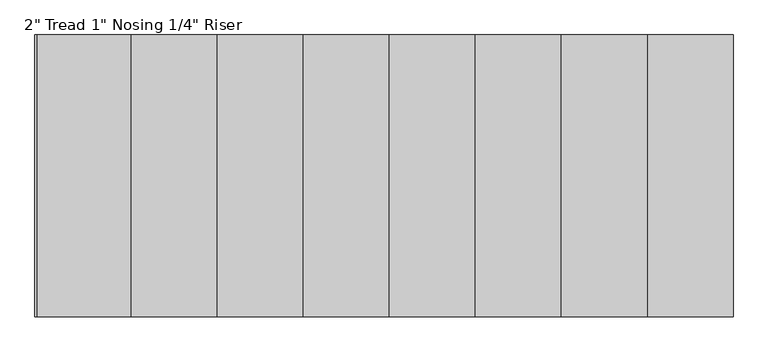
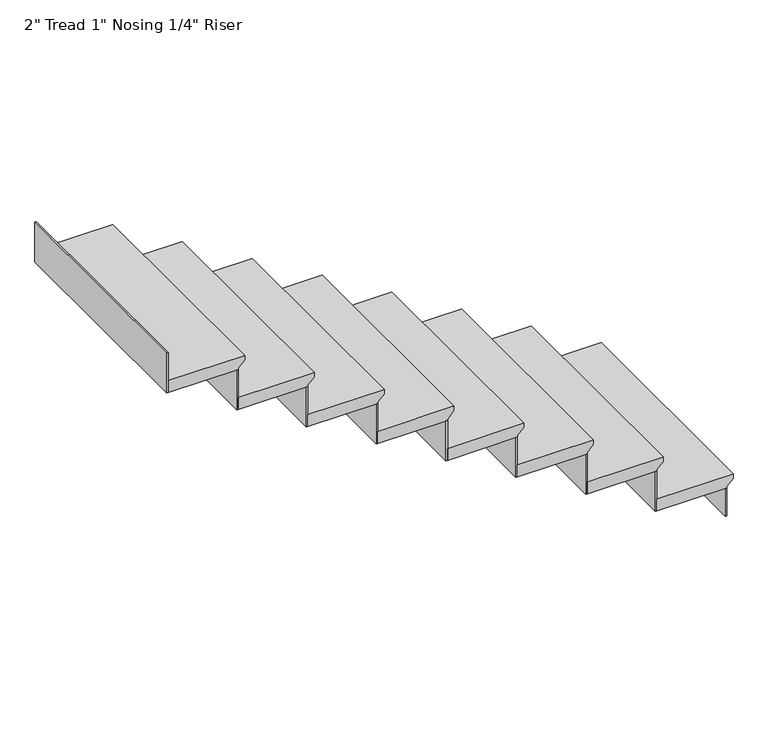
"""IFC4 building model written with IfcOpenShell, lengths in millimetres: stair flight geometry."""

from ifc_helpers import new_model, si_unit, origin, place, context, project, spatial, faceted_brep, source, transform, mapped, element, save


def stair_flight_6609341a(model_context):
    return source(origin(), model_context, "Body", "Brep", [
        faceted_brep([(-7578.3920073, 4811.1398463, 150.2833333), (-7578.3920073, 4811.1398463, 169.3333333), (-7578.3920073, 3896.7398463, 169.3333333), (-7578.3920073, 3896.7398463, 150.2833333), (-7603.7920073, 4811.1398463, 124.8833333), (-7603.7920073, 3896.7398463, 124.8833333), (-7883.1920073, 4811.1398463, 169.3333333), (-7883.1920073, 3896.7398463, 169.3333333), (-7603.7920073, 3896.7398463, 118.5333333), (-7883.1920073, 3896.7398463, 118.5333333), (-7883.1920073, 4811.1398463, 118.5333333), (-7603.7920073, 4811.1398463, 118.5333333)], [[[0, 1, 2, 3]], [[4, 0, 3, 5]], [[2, 1, 6, 7]], [[8, 9, 10, 11]], [[2, 7, 9, 8, 5, 3]], [[8, 11, 4, 5]], [[6, 1, 0, 4, 11, 10]], [[7, 6, 10, 9]]]),
        faceted_brep([(-7603.7920073, 4811.1398463, 118.5333333), (-7603.7920073, 4811.1398463, 0.0), (-7610.1420073, 4811.1398463, 0.0), (-7610.1420073, 4811.1398463, 118.5333333), (-7603.7920073, 3896.7398463, 118.5333333), (-7610.1420073, 3896.7398463, 118.5333333), (-7610.1420073, 3896.7398463, 0.0), (-7603.7920073, 3896.7398463, 0.0)], [[[0, 1, 2, 3]], [[4, 5, 6, 7]], [[1, 0, 4, 7]], [[2, 1, 7, 6]], [[3, 2, 6, 5]], [[0, 3, 5, 4]]]),
        faceted_brep([(-7883.1920073, 4811.1398463, 287.8666667), (-7883.1920073, 4811.1398463, 118.5333333), (-7889.5420073, 4811.1398463, 118.5333333), (-7889.5420073, 4811.1398463, 287.8666667), (-7883.1920073, 3896.7398463, 287.8666667), (-7889.5420073, 3896.7398463, 287.8666667), (-7889.5420073, 3896.7398463, 118.5333333), (-7883.1920073, 3896.7398463, 118.5333333)], [[[0, 1, 2, 3]], [[4, 5, 6, 7]], [[1, 0, 4, 7]], [[2, 1, 7, 6]], [[3, 2, 6, 5]], [[0, 3, 5, 4]]]),
        faceted_brep([(-7857.7920073, 3896.7398463, 338.6666667), (-7857.7920073, 4811.1398463, 338.6666667), (-8162.5920073, 4811.1398463, 338.6666667), (-8162.5920073, 3896.7398463, 338.6666667), (-7883.1920073, 3896.7398463, 287.8666667), (-8162.5920073, 3896.7398463, 287.8666667), (-8162.5920073, 4811.1398463, 287.8666667), (-7883.1920073, 4811.1398463, 287.8666667), (-7883.1920073, 3896.7398463, 294.2166667), (-7857.7920073, 3896.7398463, 319.6166667), (-7883.1920073, 4811.1398463, 294.2166667), (-7857.7920073, 4811.1398463, 319.6166667)], [[[0, 1, 2, 3]], [[4, 5, 6, 7]], [[0, 3, 5, 4, 8, 9]], [[4, 7, 10, 8]], [[2, 1, 11, 10, 7, 6]], [[3, 2, 6, 5]], [[11, 1, 0, 9]], [[10, 11, 9, 8]]]),
        faceted_brep([(-8162.5920073, 4811.1398463, 457.2), (-8162.5920073, 4811.1398463, 287.8666667), (-8168.9420073, 4811.1398463, 287.8666667), (-8168.9420073, 4811.1398463, 457.2), (-8162.5920073, 3896.7398463, 457.2), (-8168.9420073, 3896.7398463, 457.2), (-8168.9420073, 3896.7398463, 287.8666667), (-8162.5920073, 3896.7398463, 287.8666667)], [[[0, 1, 2, 3]], [[4, 5, 6, 7]], [[1, 0, 4, 7]], [[2, 1, 7, 6]], [[3, 2, 6, 5]], [[0, 3, 5, 4]]]),
        faceted_brep([(-8137.1920073, 3896.7398463, 508.0), (-8137.1920073, 4811.1398463, 508.0), (-8441.9920073, 4811.1398463, 508.0), (-8441.9920073, 3896.7398463, 508.0), (-8162.5920073, 3896.7398463, 457.2), (-8441.9920073, 3896.7398463, 457.2), (-8441.9920073, 4811.1398463, 457.2), (-8162.5920073, 4811.1398463, 457.2), (-8162.5920073, 3896.7398463, 463.55), (-8137.1920073, 3896.7398463, 488.95), (-8162.5920073, 4811.1398463, 463.55), (-8137.1920073, 4811.1398463, 488.95)], [[[0, 1, 2, 3]], [[4, 5, 6, 7]], [[0, 3, 5, 4, 8, 9]], [[4, 7, 10, 8]], [[2, 1, 11, 10, 7, 6]], [[3, 2, 6, 5]], [[11, 1, 0, 9]], [[10, 11, 9, 8]]]),
        faceted_brep([(-8441.9920073, 4811.1398463, 626.5333333), (-8441.9920073, 4811.1398463, 457.2), (-8448.3420073, 4811.1398463, 457.2), (-8448.3420073, 4811.1398463, 626.5333333), (-8441.9920073, 3896.7398463, 626.5333333), (-8448.3420073, 3896.7398463, 626.5333333), (-8448.3420073, 3896.7398463, 457.2), (-8441.9920073, 3896.7398463, 457.2)], [[[0, 1, 2, 3]], [[4, 5, 6, 7]], [[1, 0, 4, 7]], [[2, 1, 7, 6]], [[3, 2, 6, 5]], [[0, 3, 5, 4]]]),
        faceted_brep([(-8416.5920073, 3896.7398463, 677.3333333), (-8416.5920073, 4811.1398463, 677.3333333), (-8721.3920073, 4811.1398463, 677.3333333), (-8721.3920073, 3896.7398463, 677.3333333), (-8441.9920073, 3896.7398463, 626.5333333), (-8721.3920073, 3896.7398463, 626.5333333), (-8721.3920073, 4811.1398463, 626.5333333), (-8441.9920073, 4811.1398463, 626.5333333), (-8441.9920073, 3896.7398463, 632.8833333), (-8416.5920073, 3896.7398463, 658.2833333), (-8441.9920073, 4811.1398463, 632.8833333), (-8416.5920073, 4811.1398463, 658.2833333)], [[[0, 1, 2, 3]], [[4, 5, 6, 7]], [[0, 3, 5, 4, 8, 9]], [[4, 7, 10, 8]], [[2, 1, 11, 10, 7, 6]], [[3, 2, 6, 5]], [[11, 1, 0, 9]], [[10, 11, 9, 8]]]),
        faceted_brep([(-8721.3920073, 4811.1398463, 795.8666667), (-8721.3920073, 4811.1398463, 626.5333333), (-8727.7420073, 4811.1398463, 626.5333333), (-8727.7420073, 4811.1398463, 795.8666667), (-8721.3920073, 3896.7398463, 795.8666667), (-8727.7420073, 3896.7398463, 795.8666667), (-8727.7420073, 3896.7398463, 626.5333333), (-8721.3920073, 3896.7398463, 626.5333333)], [[[0, 1, 2, 3]], [[4, 5, 6, 7]], [[1, 0, 4, 7]], [[2, 1, 7, 6]], [[3, 2, 6, 5]], [[0, 3, 5, 4]]]),
        faceted_brep([(-8695.9920073, 3896.7398463, 846.6666667), (-8695.9920073, 4811.1398463, 846.6666667), (-9000.7920073, 4811.1398463, 846.6666667), (-9000.7920073, 3896.7398463, 846.6666667), (-8721.3920073, 3896.7398463, 795.8666667), (-9000.7920073, 3896.7398463, 795.8666667), (-9000.7920073, 4811.1398463, 795.8666667), (-8721.3920073, 4811.1398463, 795.8666667), (-8721.3920073, 3896.7398463, 802.2166667), (-8695.9920073, 3896.7398463, 827.6166667), (-8721.3920073, 4811.1398463, 802.2166667), (-8695.9920073, 4811.1398463, 827.6166667)], [[[0, 1, 2, 3]], [[4, 5, 6, 7]], [[0, 3, 5, 4, 8, 9]], [[4, 7, 10, 8]], [[2, 1, 11, 10, 7, 6]], [[3, 2, 6, 5]], [[11, 1, 0, 9]], [[10, 11, 9, 8]]]),
        faceted_brep([(-9000.7920073, 4811.1398463, 965.2), (-9000.7920073, 4811.1398463, 795.8666667), (-9007.1420073, 4811.1398463, 795.8666667), (-9007.1420073, 4811.1398463, 965.2), (-9000.7920073, 3896.7398463, 965.2), (-9007.1420073, 3896.7398463, 965.2), (-9007.1420073, 3896.7398463, 795.8666667), (-9000.7920073, 3896.7398463, 795.8666667)], [[[0, 1, 2, 3]], [[4, 5, 6, 7]], [[1, 0, 4, 7]], [[2, 1, 7, 6]], [[3, 2, 6, 5]], [[0, 3, 5, 4]]]),
        faceted_brep([(-8975.3920073, 3896.7398463, 1016.0), (-8975.3920073, 4811.1398463, 1016.0), (-9280.1920073, 4811.1398463, 1016.0), (-9280.1920073, 3896.7398463, 1016.0), (-9000.7920073, 3896.7398463, 965.2), (-9280.1920073, 3896.7398463, 965.2), (-9280.1920073, 4811.1398463, 965.2), (-9000.7920073, 4811.1398463, 965.2), (-9000.7920073, 3896.7398463, 971.55), (-8975.3920073, 3896.7398463, 996.95), (-9000.7920073, 4811.1398463, 971.55), (-8975.3920073, 4811.1398463, 996.95)], [[[0, 1, 2, 3]], [[4, 5, 6, 7]], [[0, 3, 5, 4, 8, 9]], [[4, 7, 10, 8]], [[2, 1, 11, 10, 7, 6]], [[3, 2, 6, 5]], [[11, 1, 0, 9]], [[10, 11, 9, 8]]]),
        faceted_brep([(-9280.1920073, 4811.1398463, 1134.5333333), (-9280.1920073, 4811.1398463, 965.2), (-9286.5420073, 4811.1398463, 965.2), (-9286.5420073, 4811.1398463, 1134.5333333), (-9280.1920073, 3896.7398463, 1134.5333333), (-9286.5420073, 3896.7398463, 1134.5333333), (-9286.5420073, 3896.7398463, 965.2), (-9280.1920073, 3896.7398463, 965.2)], [[[0, 1, 2, 3]], [[4, 5, 6, 7]], [[1, 0, 4, 7]], [[2, 1, 7, 6]], [[3, 2, 6, 5]], [[0, 3, 5, 4]]]),
        faceted_brep([(-9254.7920073, 3896.7398463, 1185.3333333), (-9254.7920073, 4811.1398463, 1185.3333333), (-9559.5920073, 4811.1398463, 1185.3333333), (-9559.5920073, 3896.7398463, 1185.3333333), (-9280.1920073, 3896.7398463, 1134.5333333), (-9559.5920073, 3896.7398463, 1134.5333333), (-9559.5920073, 4811.1398463, 1134.5333333), (-9280.1920073, 4811.1398463, 1134.5333333), (-9280.1920073, 3896.7398463, 1140.8833333), (-9254.7920073, 3896.7398463, 1166.2833333), (-9280.1920073, 4811.1398463, 1140.8833333), (-9254.7920073, 4811.1398463, 1166.2833333)], [[[0, 1, 2, 3]], [[4, 5, 6, 7]], [[0, 3, 5, 4, 8, 9]], [[4, 7, 10, 8]], [[2, 1, 11, 10, 7, 6]], [[3, 2, 6, 5]], [[11, 1, 0, 9]], [[10, 11, 9, 8]]]),
        faceted_brep([(-9838.9920073, 4811.1398463, 1473.2), (-9838.9920073, 4811.1398463, 1303.8666667), (-9845.3420073, 4811.1398463, 1303.8666667), (-9845.3420073, 4811.1398463, 1473.2), (-9838.9920073, 3896.7398463, 1473.2), (-9845.3420073, 3896.7398463, 1473.2), (-9845.3420073, 3896.7398463, 1303.8666667), (-9838.9920073, 3896.7398463, 1303.8666667)], [[[0, 1, 2, 3]], [[4, 5, 6, 7]], [[1, 0, 4, 7]], [[2, 1, 7, 6]], [[3, 2, 6, 5]], [[0, 3, 5, 4]]]),
        faceted_brep([(-9559.5920073, 4811.1398463, 1303.8666667), (-9559.5920073, 4811.1398463, 1134.5333333), (-9565.9420073, 4811.1398463, 1134.5333333), (-9565.9420073, 4811.1398463, 1303.8666667), (-9559.5920073, 3896.7398463, 1303.8666667), (-9565.9420073, 3896.7398463, 1303.8666667), (-9565.9420073, 3896.7398463, 1134.5333333), (-9559.5920073, 3896.7398463, 1134.5333333)], [[[0, 1, 2, 3]], [[4, 5, 6, 7]], [[1, 0, 4, 7]], [[2, 1, 7, 6]], [[3, 2, 6, 5]], [[0, 3, 5, 4]]]),
        faceted_brep([(-9534.1920073, 3896.7398463, 1354.6666667), (-9534.1920073, 4811.1398463, 1354.6666667), (-9813.5920073, 4811.1398463, 1354.6666667), (-9838.9920073, 4811.1398463, 1354.6666667), (-9838.9920073, 3896.7398463, 1354.6666667), (-9559.5920073, 3896.7398463, 1303.8666667), (-9838.9920073, 3896.7398463, 1303.8666667), (-9838.9920073, 4811.1398463, 1303.8666667), (-9813.5920073, 4811.1398463, 1303.8666667), (-9559.5920073, 4811.1398463, 1303.8666667), (-9559.5920073, 3896.7398463, 1310.2166667), (-9534.1920073, 3896.7398463, 1335.6166667), (-9559.5920073, 4811.1398463, 1310.2166667), (-9534.1920073, 4811.1398463, 1335.6166667)], [[[0, 1, 2, 3, 4]], [[5, 6, 7, 8, 9]], [[0, 4, 6, 5, 10, 11]], [[5, 9, 12, 10]], [[2, 1, 13, 12, 9, 8]], [[3, 2, 8, 7]], [[4, 3, 7, 6]], [[13, 1, 0, 11]], [[12, 13, 11, 10]]]),
    ])


if __name__ == "__main__":
    model = new_model("IFC4")
    model_context = context("Model", 3, world=origin())
    ifc_project = project(units=[si_unit("LENGTHUNIT", "METRE", prefix="MILLI")], contexts=[model_context])
    site = spatial("IfcSite", under=ifc_project)
    building = spatial("IfcBuilding", under=site)
    placement = place(None, origin())
    stair_flight_shape = stair_flight_6609341a(model_context)
    element("IfcStairFlight", 1, ObjectType="2\" Tread 1\" Nosing 1/4\" Riser", at=placement, inside=building, context=model_context, shape_type="MappedRepresentation", body=[
        mapped(stair_flight_shape, transform((0.0, 0.0, 0.0), x_axis=(1.0, 0.0, 0.0), y_axis=(0.0, 1.0, 0.0), z_axis=(0.0, 0.0, 1.0))),
    ])
    save(model, "model.ifc")
